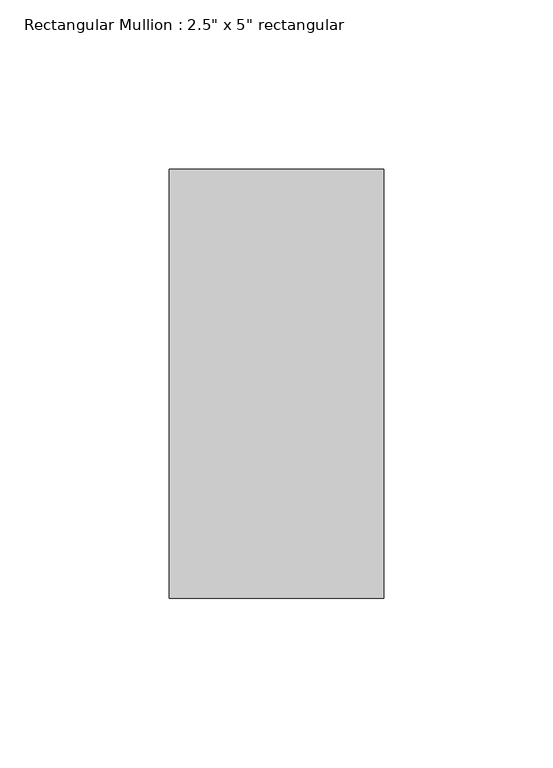
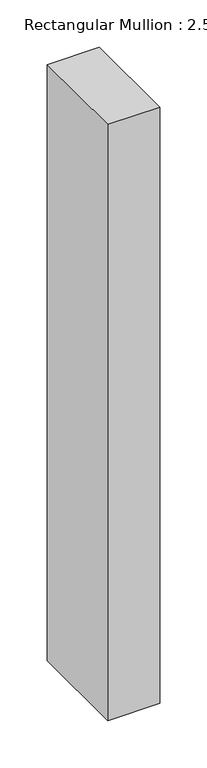
"""IFC4 building model written with IfcOpenShell, lengths in millimetres: member geometry."""

from ifc_helpers import new_model, si_unit, frame, origin, place, context, project, spatial, polyline, outline, extrude, source, transform, mapped, element, save


def member_7d5d45fc(model_context):
    return source(origin(), model_context, "Body", "SweptSolid", [
        extrude(outline(polyline([(31.75, 63.5), (31.75, -63.5), (-31.75, -63.5), (-31.75, 63.5), (31.75, 63.5)])), frame((0.0, 0.0, -768.35), z_axis=(0.0, 0.0, 1.0), x_axis=(1.0, 0.0, 0.0)), (0.0, 0.0, 1.0), 768.35),
    ])


if __name__ == "__main__":
    model = new_model("IFC4")
    model_context = context("Model", 3, world=origin())
    ifc_project = project(units=[si_unit("LENGTHUNIT", "METRE", prefix="MILLI")], contexts=[model_context])
    site = spatial("IfcSite", under=ifc_project)
    building = spatial("IfcBuilding", under=site)
    placement = place(None, origin())
    member_shape = member_7d5d45fc(model_context)
    element("IfcMember", 1, ObjectType="Rectangular Mullion : 2.5\" x 5\" rectangular", at=placement, inside=building, context=model_context, shape_type="MappedRepresentation", body=[
        mapped(member_shape, transform((0.0, 0.0, 0.0), x_axis=(1.0, 0.0, 0.0), y_axis=(0.0, 1.0, 0.0), z_axis=(0.0, 0.0, 1.0))),
    ])
    save(model, "model.ifc")

# Revit data of these elements
# Type "Rectangular Mullion : 2.5\" x 5\" rectangular"
#   built-in parameter 1007304 = 0.416667 (stored number, unit not read)
#   built-in parameter 1007301 = 0.104167 (stored number, unit not read)
#   built-in parameter 1007300 = 0.104167 (stored number, unit not read)
# Element 1 (IfcMember, "Rectangular Mullion : 2.5\" x 5\" rectangular")
#   Materials on its faces: "Aluminum"
# Materials
#   "Aluminum": class "Metal", colour RGB 247 247 247, transparency 0, Description = "Aluminum 6061", Cost = 0
